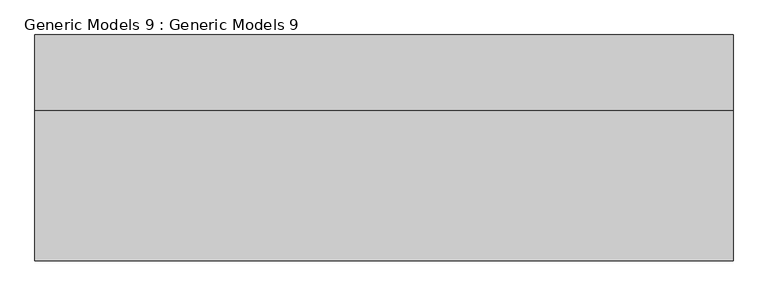
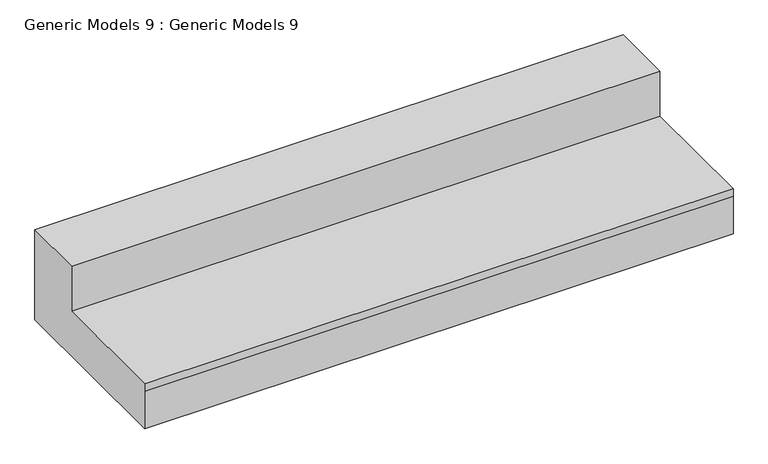
"""IFC4 building model written with IfcOpenShell, lengths in millimetres: proxy geometry, Generic Models 9 : Generic Models 9."""

from ifc_helpers import new_model, si_unit, frame, origin, place, context, project, spatial, polyline, outline, extrude, source, transform, mapped, element, save


def generic_models_9_generic_models_9_d0116728(model_context):
    return source(origin(), model_context, "Body", "SweptSolid", [
        extrude(outline(polyline([(-4272.2938352, 0.0), (-4881.8938352, 0.0), (-4881.8938352, 127.0), (-4881.8938352, 152.4), (-4475.4938352, 152.4), (-4475.4938352, 304.8), (-4272.2938352, 304.8), (-4272.2938352, 0.0)])), frame((-421.8231182, 0.0, 0.0), z_axis=(1.0, 0.0, 0.0), x_axis=(0.0, 1.0, 0.0)), (0.0, 0.0, 1.0), 1885.8400881),
    ])


if __name__ == "__main__":
    model = new_model("IFC4")
    model_context = context("Model", 3, world=origin())
    ifc_project = project(units=[si_unit("LENGTHUNIT", "METRE", prefix="MILLI")], contexts=[model_context])
    site = spatial("IfcSite", under=ifc_project)
    building = spatial("IfcBuilding", under=site)
    placement = place(None, origin())
    generic_models_9_generic_models_9_shape = generic_models_9_generic_models_9_d0116728(model_context)
    element("IfcBuildingElementProxy", 1, Name="Generic Models 9 : Generic Models 9", ObjectType="Generic Models 9 : Generic Models 9", at=placement, inside=building, context=model_context, shape_type="MappedRepresentation", body=[
        mapped(generic_models_9_generic_models_9_shape, transform((0.0, 0.0, 0.0), x_axis=(1.0, 0.0, 0.0), y_axis=(0.0, 1.0, 0.0), z_axis=(0.0, 0.0, 1.0))),
    ])
    save(model, "model.ifc")

# Revit data of these elements
# Element 1 (IfcBuildingElementProxy, "Generic Models 9 : Generic Models 9")
#   Materials on its faces: "Concrete, Cast-in-Place gray"
# Materials
#   "Concrete, Cast-in-Place gray": class "Concrete", colour RGB 192 192 192, transparency 0, Description = "Cast-in-place concrete", Cost = 0
